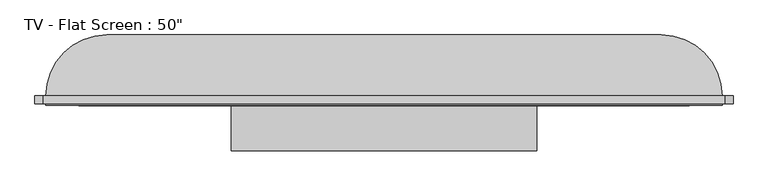
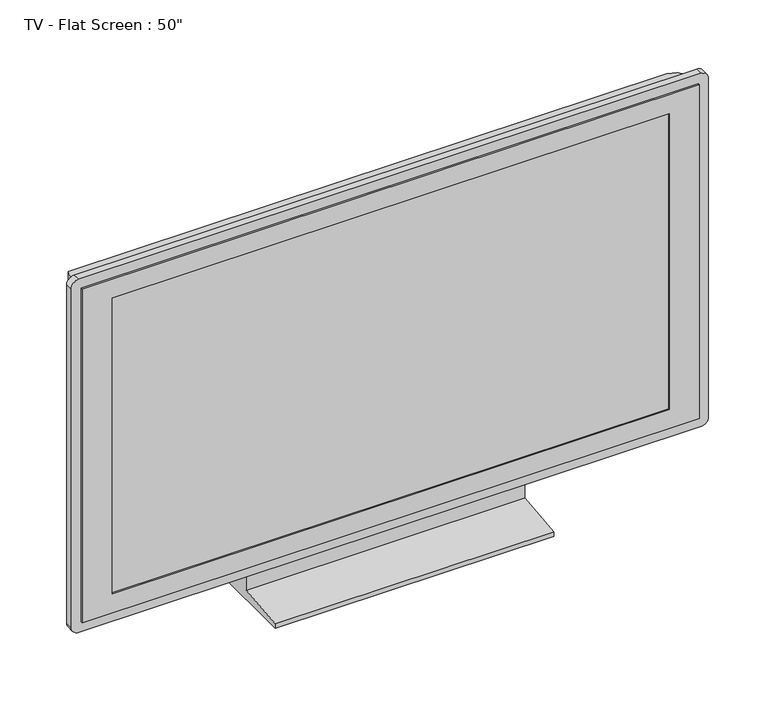
"""IFC4 building model written with IfcOpenShell, lengths in millimetres: furniture geometry."""

from ifc_helpers import new_model, si_unit, point, frame, frame_2d, origin, place, context, project, spatial, polyline, circle_curve, ellipse_curve, trimmed, segment, composite_curve, outline, extrude, faceted_brep, source, transform, mapped, element, save
from ifc_brep_helpers import plane_surface, cylinder_surface, advanced_brep


def furniture_0b81fedb(model_context):
    return source(origin(), model_context, "Body", "SolidModel", [
        advanced_brep(
        [(-617.3827737, -51.4613764, 80.0), (609.4937454, -51.4613764, 80.0), (609.4937454, -51.4613764, 782.6751733), (-617.3827737, -51.4613764, 782.6751733), (499.4937454, 58.5386236, 80.0), (-507.3827737, 58.5386236, 80.0), (-507.3827737, 58.5386236, 672.6751733), (499.4937454, 58.5386236, 672.6751733)],
        [
            (0, 1),
            (1, 2),
            (2, 3),
            (3, 0),
            (4, 5),
            (5, 6),
            (6, 7),
            (7, 4),
            (0, 5, circle_curve(frame((-507.3827737, -51.4613764, 80.0), z_axis=(0.0, 0.0, -1.0), x_axis=(-1.0, 0.0, 0.0)), 110.0)),
            (4, 1, circle_curve(frame((499.4937454, -51.4613764, 80.0), z_axis=(0.0, 0.0, -1.0), x_axis=(1.0, 0.0, 0.0)), 110.0)),
            (7, 2, ellipse_curve(frame((499.4937454, -51.4613764, 672.6751733), z_axis=(0.7071067811865475, 0.0, -0.7071067811865475), x_axis=(0.7071067811865474, 0.0, 0.7071067811865476)), 155.5634919, 110.0)),
            (6, 3, ellipse_curve(frame((-507.3827737, -51.4613764, 672.6751733), z_axis=(0.7071067811865475, 0.0, 0.7071067811865475), x_axis=(-0.7071067811865476, 0.0, 0.7071067811865474)), 155.5634919, 110.0)),
        ],
        [
            plane_surface(frame((-617.3827737, -51.4613764, 782.6751733), z_axis=(0.0, -1.0, 0.0), x_axis=(-1.0, 0.0, 0.0))),
            plane_surface(frame((-617.3827737, 58.5386236, 782.6751733), z_axis=(0.0, 1.0, 0.0), x_axis=(1.0, 0.0, 0.0))),
            plane_surface(frame((-617.3827737, -51.4613764, 80.0), z_axis=(0.0, 0.0, -1.0), x_axis=(0.0, 1.0, 0.0))),
            cylinder_surface(frame((499.4937454, -51.4613764, 80.0), z_axis=(0.0, 0.0, 1.0), x_axis=(1.0, 0.0, 0.0)), 110.0),
            cylinder_surface(frame((609.4937454, -51.4613764, 672.6751733), z_axis=(-1.0, 0.0, 0.0), x_axis=(0.0, 0.0, 1.0)), 110.0),
            cylinder_surface(frame((-507.3827737, -51.4613764, 782.6751733), z_axis=(0.0, 0.0, -1.0), x_axis=(-1.0, 0.0, 0.0)), 110.0),
        ],
        [
            (0, [[1, 2, 3, 4]]),
            (1, [[5, 6, 7, 8]]),
            (2, [[-1, 9, -5, 10]]),
            (3, [[11, -2, -10, -8]]),
            (4, [[-11, -7, 12, -3]]),
            (5, [[-12, -6, -9, -4]]),
        ],
    ),
        extrude(outline(composite_curve([segment(polyline([(802.6751733, 614.4937454), (802.6751733, -622.3827737)]), True, "CONTINUOUS"), segment(trimmed(circle_curve(frame_2d((787.6751733, -622.3827737)), 15.0), [point((802.6751733, -622.3827737))], [point((787.6751733, -637.3827737))], False, "CARTESIAN"), True, "CONTINUOUS"), segment(polyline([(787.6751733, -637.3827737), (75.0, -637.3827737)]), True, "CONTINUOUS"), segment(trimmed(circle_curve(frame_2d((75.0, -622.3827737)), 15.0), [point((75.0, -637.3827737))], [point((60.0, -622.3827737))], False, "CARTESIAN"), True, "CONTINUOUS"), segment(polyline([(60.0, -622.3827737), (60.0, 614.4937454)]), True, "CONTINUOUS"), segment(trimmed(circle_curve(frame_2d((75.0, 614.4937454)), 15.0), [point((60.0, 614.4937454))], [point((75.0, 629.4937454))], False, "CARTESIAN"), True, "CONTINUOUS"), segment(polyline([(75.0, 629.4937454), (787.6751733, 629.4937454)]), True, "CONTINUOUS"), segment(trimmed(circle_curve(frame_2d((787.6751733, 614.4937454)), 15.0), [point((787.6751733, 629.4937454))], [point((802.6751733, 614.4937454))], False, "CARTESIAN"), True, "CONTINUOUS")], self_intersect=False), holes=[polyline([(782.6751733, 609.4937454), (80.0, 609.4937454), (80.0, -617.3827737), (782.6751733, -617.3827737), (782.6751733, 609.4937454)])]), frame((0.0, -66.4613764, 0.0), z_axis=(0.0, 1.0, 0.0), x_axis=(0.0, 0.0, 1.0)), (0.0, 0.0, 1.0), 15.0),
        faceted_brep([(609.4937454, -69.4613764, 782.6751733), (-617.3827737, -69.4613764, 782.6751733), (-617.3827737, -69.4613764, 80.0), (609.4937454, -69.4613764, 80.0), (-557.3827737, -69.4613764, 742.6751733), (549.4937454, -69.4613764, 742.6751733), (549.4937454, -69.4613764, 120.0), (-557.3827737, -69.4613764, 120.0), (609.4937454, -51.4613764, 782.6751733), (609.4937454, -51.4613764, 80.0), (-617.3827737, -51.4613764, 80.0), (-617.3827737, -51.4613764, 782.6751733), (-557.3827737, -66.4613764, 742.6751733), (-557.3827737, -66.4613764, 120.0), (549.4937454, -66.4613764, 120.0), (549.4937454, -66.4613764, 742.6751733)], [[[0, 1, 2, 3], [4, 5, 6, 7]], [[8, 9, 10, 11]], [[1, 0, 8, 11]], [[2, 1, 11, 10]], [[3, 2, 10, 9]], [[0, 3, 9, 8]], [[12, 13, 14, 15]], [[12, 15, 5, 4]], [[15, 14, 6, 5]], [[14, 13, 7, 6]], [[13, 12, 4, 7]]]),
        extrude(outline(polyline([(-51.4613764, 80.0), (-1.4613764, 80.0), (48.5386236, 0.0), (-151.4613764, 0.0), (-151.4613764, 10.0), (-51.4613764, 20.0), (-51.4613764, 80.0)])), frame((-280.6636439, 0.0, 0.0), z_axis=(1.0, 0.0, 0.0), x_axis=(0.0, 1.0, 0.0)), (0.0, 0.0, 1.0), 553.4382596),
    ])


if __name__ == "__main__":
    model = new_model("IFC4")
    model_context = context("Model", 3, world=origin())
    ifc_project = project(units=[si_unit("LENGTHUNIT", "METRE", prefix="MILLI")], contexts=[model_context])
    site = spatial("IfcSite", under=ifc_project)
    building = spatial("IfcBuilding", under=site)
    placement = place(None, origin())
    furniture_shape = furniture_0b81fedb(model_context)
    element("IfcFurniture", 1, ObjectType="TV - Flat Screen : 50\"", at=placement, inside=building, context=model_context, shape_type="MappedRepresentation", body=[
        mapped(furniture_shape, transform((0.0, 0.0, 0.0), x_axis=(1.0, 0.0, 0.0), y_axis=(0.0, 1.0, 0.0), z_axis=(0.0, 0.0, 1.0))),
    ])
    save(model, "model.ifc")

# Revit data of these elements
# Type "TV - Flat Screen : 50\""
#   SinAng = 0' - 0.0193"
#   L = 3' - 7.57782"
#   H = 2' - 0.51477"
#   Thickness = 0' - 4.33071"
#   Diagonal = 4' - 2"
#   CosAng = 0' - 0.03431"
#   Stand [instance default] = yes
#   Default Elevation = 0
# Element 1 (IfcFurniture, "TV - Flat Screen : 50\"")
#   Materials on its faces: "TV - Black", "TV - Glass", "TV - Screen"
# Materials
#   "TV - Black": colour RGB 49 49 49, transparency 0
#   "TV - Glass": colour RGB 157 157 157, transparency 0.9
#   "TV - Screen": colour RGB 0 0 0, transparency 0
